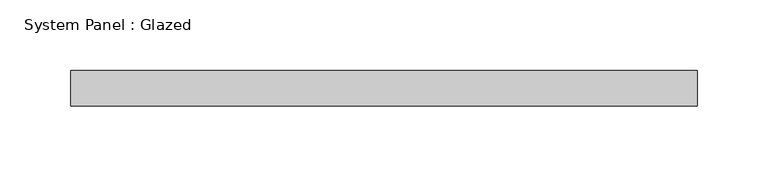
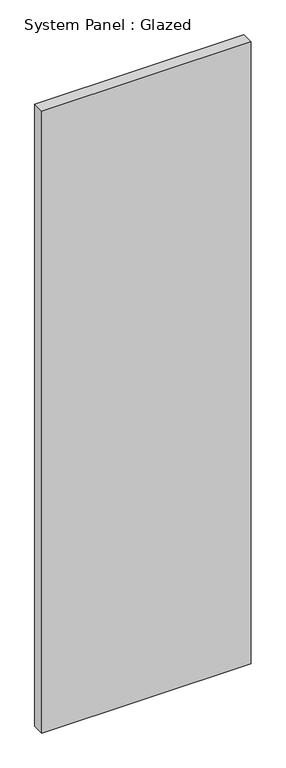
"""IFC4 building model written with IfcOpenShell, lengths in millimetres: plate geometry, System Panel : Glazed."""

from ifc_helpers import new_model, si_unit, origin, origin_with_axes, place, context, project, spatial, polyline, outline, extrude, source, transform, mapped, element, save


def system_panel_glazed_fa064951(model_context):
    return source(origin(), model_context, "Body", "SweptSolid", [
        extrude(outline(polyline([(222.25, 19.05), (-222.25, 19.05), (-222.25, 44.45), (222.25, 44.45), (222.25, 19.05)])), origin_with_axes(), (0.0, 0.0, 1.0), 1395.1457324),
    ])


if __name__ == "__main__":
    model = new_model("IFC4")
    model_context = context("Model", 3, world=origin())
    ifc_project = project(units=[si_unit("LENGTHUNIT", "METRE", prefix="MILLI")], contexts=[model_context])
    site = spatial("IfcSite", under=ifc_project)
    building = spatial("IfcBuilding", under=site)
    placement = place(None, origin())
    system_panel_glazed_shape = system_panel_glazed_fa064951(model_context)
    element("IfcPlate", 1, ObjectType="System Panel : Glazed", at=placement, inside=building, context=model_context, shape_type="MappedRepresentation", body=[
        mapped(system_panel_glazed_shape, transform((0.0, 0.0, 0.0), x_axis=(1.0, 0.0, 0.0), y_axis=(0.0, 1.0, 0.0), z_axis=(0.0, 0.0, 1.0))),
    ])
    save(model, "model.ifc")

# Revit data of these elements
# Type "System Panel : Glazed"
#   Construction Type Id = "GSP4R"
#   Analytic Construction = "1/8 in Pilkington single glazing"
#   Visual Light Transmittance = 0.9
#   Solar Heat Gain Coefficient = 0.86
#   Heat Transfer Coefficient (U) = 1.18115 BTU/(h·ft²·°F)
#   Define Thermal Properties by = 1
# Element 1 (IfcPlate, "System Panel : Glazed")
#   Materials on its faces: "Glass"
# Materials
#   "Glass": class "Glass", colour RGB 0 128 192, transparency 0.75, Description = "Soda Lime Glass", Cost = 0
